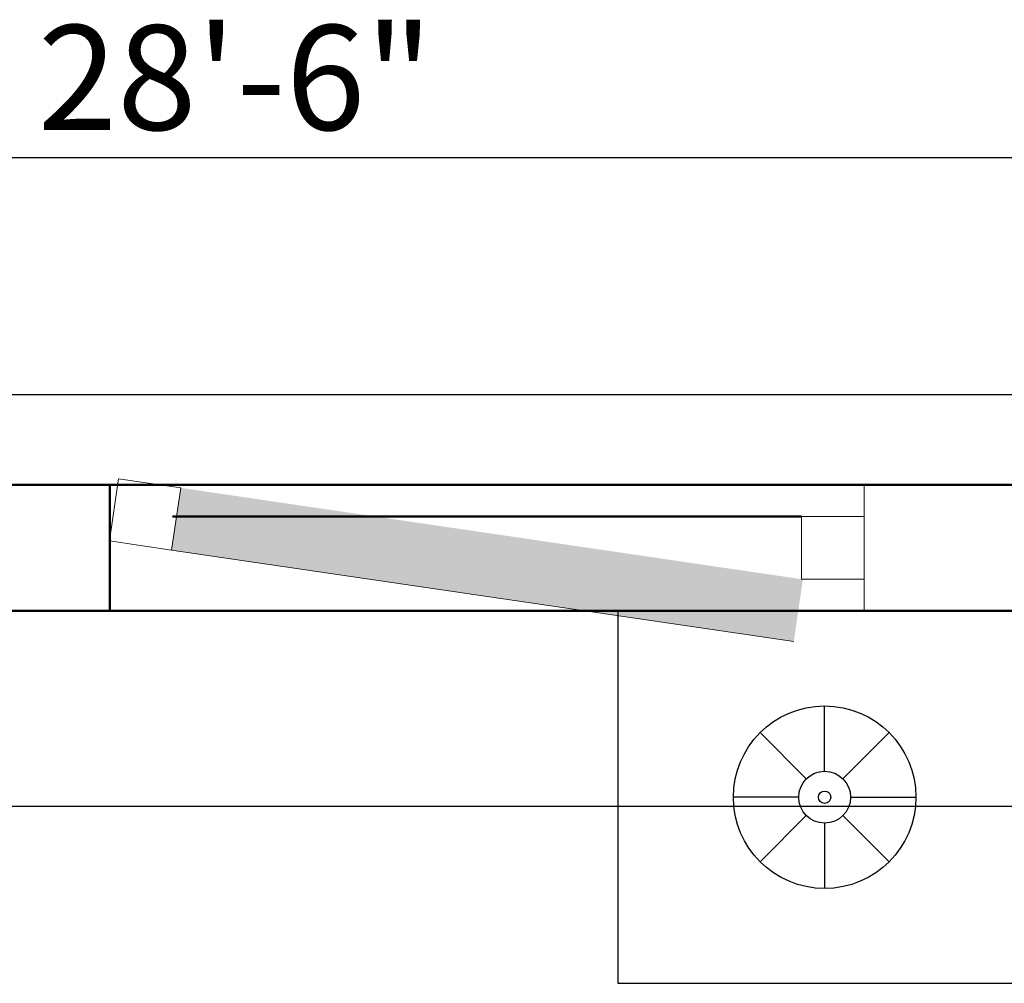
# Model space of a CAD drawing. Units: inches. Extents: x 3064 to 19385, y 846 to 15425.
# Tile 103 of 108: x 7687 to 7734, y 1373 to 1419. Entities that reach past the tile are written whole.
import ezdxf

# ---------------------------------------------------------------- set-up
doc = ezdxf.new("R2010")
doc.units = ezdxf.units.IN
for name, color, linetype, lineweight in [('A-ANNO-DIMS', 2, 'Continuous', 18), ('A-FLOR-FIXT', 9, 'Continuous', 18), ('A-GLAZ', 4, 'Continuous', 18), ('A-WALL', 7, 'Continuous', 50)]:
    doc.layers.add(name, color=color, linetype=linetype, lineweight=lineweight)
doc.layers.add('BLOCK', color=6, linetype='Continuous')
doc.styles.get("Standard").update_dxf_attribs({"font": 'arial.ttf'})
doc.dimstyles.new('ISO-25', dxfattribs={"dimtxt": 9, "dimasz": 2.5, "dimexe": 1.25, "dimexo": 0.625, "dimtad": 1, "dimdec": 1, "dimlunit": 3, "dimtxsty": 'Standard', "dimcen": 2.5, "dimadec": 0, "dimazin": 0, "dimtfac": 1, "dimtdec": 1, "dimtmove": 0, "dimatfit": 3, "dimfxl": 1, "dimarcsym": 0})

# ---------------------------------------------------------------- blocks, each defined once
blk = doc.blocks.new('*D338')
at = {"layer": 'A-ANNO-DIMS', "color": 0, "lineweight": -2, "transparency": 16777216}
for p, q in [((7667.246, 1396.965), (7667.246, 1401.902)), ((7862.246, 1396.965), (7862.246, 1401.902)), ((7669.746, 1400.652), (7859.746, 1400.652))]:
    blk.add_line(p, q, dxfattribs=at)
at = {"layer": 'A-ANNO-DIMS', "color": 0, "transparency": 16777216}
for points in [[(7669.746, 1401.069), (7669.746, 1400.235), (7667.246, 1400.652)], [(7859.746, 1401.069), (7859.746, 1400.235), (7862.246, 1400.652)]]:
    blk.add_solid(points, dxfattribs=at)
at = {"layer": 'Defpoints', "color": 0, "transparency": 16777216}
for p in [(7862.246, 1400.652), (7667.246, 1396.34), (7862.246, 1396.34)]:
    blk.add_point(p, dxfattribs=at)
at = {"layer": 'A-ANNO-DIMS', "color": 0, "transparency": 16777216, "insert": (7764.746, 1403.832), "char_height": 5, "attachment_point": 5}
blk.add_mtext('16\'-3"', dxfattribs=at)
blk = doc.blocks.new('*D226')
at = {"layer": 'A-ANNO-DIMS', "color": 0, "lineweight": -2, "transparency": 16777216}
for p, q in [((7526.246, 1396.965), (7526.246, 1413.199)), ((7868.246, 1396.965), (7868.246, 1413.199)), ((7865.746, 1411.949), (7528.746, 1411.949))]:
    blk.add_line(p, q, dxfattribs=at)
at = {"layer": 'A-ANNO-DIMS', "color": 0, "transparency": 16777216}
for points in [[(7528.746, 1412.366), (7528.746, 1411.533), (7526.246, 1411.949)], [(7865.746, 1412.366), (7865.746, 1411.533), (7868.246, 1411.949)]]:
    blk.add_solid(points, dxfattribs=at)
at = {"layer": 'Defpoints', "color": 0, "transparency": 16777216}
for p in [(7526.246, 1411.949), (7526.246, 1396.34), (7868.246, 1396.34)]:
    blk.add_point(p, dxfattribs=at)
at = {"layer": 'A-ANNO-DIMS', "color": 0, "transparency": 16777216, "insert": (7697.246, 1415.127), "char_height": 5, "attachment_point": 5}
blk.add_mtext('28\'-6"', dxfattribs=at)
blk = doc.blocks.new('*D248')
at = {"layer": 'A-ANNO-DIMS', "color": 0, "lineweight": -2, "transparency": 16777216}
for p, q in [((7667.246, 1389.715), (7667.246, 1379.771)), ((7862.246, 1389.715), (7862.246, 1379.771)), ((7669.746, 1381.021), (7859.746, 1381.021))]:
    blk.add_line(p, q, dxfattribs=at)
at = {"layer": 'A-ANNO-DIMS', "color": 0, "transparency": 16777216}
for points in [[(7669.746, 1381.437), (7669.746, 1380.604), (7667.246, 1381.021)], [(7859.746, 1381.437), (7859.746, 1380.604), (7862.246, 1381.021)]]:
    blk.add_solid(points, dxfattribs=at)
at = {"layer": 'Defpoints', "color": 0, "transparency": 16777216}
for p in [(7667.246, 1390.34), (7862.246, 1390.34), (7862.246, 1381.021)]:
    blk.add_point(p, dxfattribs=at)
at = {"layer": 'A-ANNO-DIMS', "color": 0, "transparency": 16777216, "insert": (7764.746, 1384.2), "char_height": 5, "attachment_point": 5}
blk.add_mtext('16\'-3"', dxfattribs=at)
blk = doc.blocks.new('A$C52E67D0D')
at = {"layer": 'BLOCK'}
for p, q in [((250.5, 1605.5), (250.5, 1684.7)), ((228.3, 1596.3), (172.3, 1652.3)), ((272.7, 1596.3), (328.7, 1652.3)), ((219.1, 1574.1), (139.9, 1574.1)), ((281.9, 1574.1), (361.1, 1574.1)), ((228.3, 1551.9), (172.3, 1495.9)), ((272.7, 1551.9), (328.7, 1495.9)), ((250.5, 1542.8), (250.5, 1463.5))]:
    blk.add_line(p, q, dxfattribs=at)
blk.add_lwpolyline([(501, 1348.6), (501, 1799.6), (0, 1799.6), (0, 1348.6)], close=True, dxfattribs=at)
for radius in [110.6, 31.4, 7.46]:
    blk.add_circle((250.5, 1574.1), radius, dxfattribs=at)
blk = doc.blocks.new('WIN-900-A')
h = blk.add_hatch(color=256)
h.dxf.hatch_style = 1
h.paths.add_polyline_path([(33, 0), (33, 3), (3, 3), (3, 0)])
blk.add_line((3, 0), (33, 0))
blk.add_lwpolyline([(3, 0), (0, 0), (0, 3), (3, 3)], close=True)

msp = doc.modelspace()

# ---------------------------------------------------------------- linework, layer by layer
at = {"layer": 'A-GLAZ'}
msp.add_line((7727.246, 1396.34), (7727.246, 1390.34), dxfattribs=at)
msp.add_lwpolyline([(7727.246, 1391.84), (7724.246, 1391.84), (7724.246, 1394.84), (7727.246, 1394.84)], close=True, dxfattribs=at)
at = {"layer": 'A-WALL'}
for p, q in [((7868.246, 1396.34), (7526.246, 1396.34)), ((7691.246, 1396.34), (7691.246, 1390.34)), ((7694.246, 1394.84), (7724.246, 1394.84)), ((7862.246, 1390.34), (7667.246, 1390.34))]:
    msp.add_line(p, q, dxfattribs=at)

# ---------------------------------------------------------------- block references
at = {"layer": 'A-FLOR-FIXT', "xscale": 0.039370099999992, "yscale": 0.039370099999992, "zscale": 0.039370099999992}
msp.add_blockref('A$C52E67D0D', (7715.494, 1319.474), dxfattribs=at)
at = {"layer": 'A-GLAZ', "rotation": 351.6350998303229}
msp.add_blockref('WIN-900-A', (7691.233, 1393.669), dxfattribs=at)

# ---------------------------------------------------------------- dimensions: what is measured, and where the dimension line sits
at = {"layer": 'A-ANNO-DIMS'}
for base, p1, p2, override, picture, middle in [((7526.246, 1411.949), (7868.246, 1396.34), (7526.246, 1396.34), {"dimtxt": 5, "dimclrd": 0, "dimclre": 0, "dimclrt": 0}, '*D226', (7697.246, 1415.127)), ((7862.246, 1400.652), (7667.246, 1396.34), (7862.246, 1396.34), {"dimtxt": 5, "dimclrd": 0, "dimclre": 0, "dimclrt": 0, "dimtmove": 1}, '*D338', (7764.746, 1403.832)), ((7862.246, 1381.021), (7667.246, 1390.34), (7862.246, 1390.34), {"dimtxt": 5, "dimclrd": 0, "dimclre": 0, "dimclrt": 0}, '*D248', (7764.746, 1384.2))]:
    dim = msp.add_linear_dim(base=base, p1=p1, p2=p2, dimstyle='ISO-25', override=override, dxfattribs=at)
    dim.commit()
    dim.dimension.update_dxf_attribs({"geometry": picture, "text_midpoint": middle})

doc.saveas('drawing.dxf')
